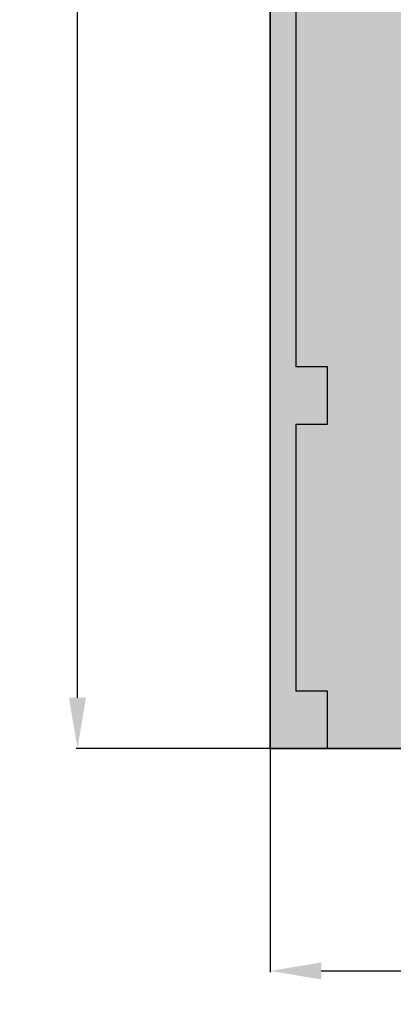
# Model space of a CAD drawing. Units: inches. Extents: x 389 to 971, y 148 to 870.
# Tile 1 of 14: x 389 to 448, y 194 to 349. Entities that reach past the tile are written whole.
import ezdxf

# ---------------------------------------------------------------- set-up
doc = ezdxf.new("R2010")
doc.units = ezdxf.units.IN
doc.header["$MEASUREMENT"] = 0
for name, color, linetype, lineweight in [('A-ANNO-DIMS', 2, 'Continuous', 18), ('C-PROP', 7, 'Continuous', 35), ('L-GATE', 4, 'Continuous', 25), ('L-GRND-BASE-PATT', 8, 'Continuous', 13), ('L-WALL', 7, 'Continuous', 30)]:
    doc.layers.add(name, color=color, linetype=linetype, lineweight=lineweight)
for name, color, linetype, lineweight, true_color in [('A-WALL-PATT', 18, 'Continuous', 13, 0x000000), ('L-GRND-PATT', 39, 'Continuous', 13, 0x603913), ('L-WALL-PATT', 18, 'Continuous', 13, 0x000000)]:
    doc.layers.add(name, color=color, linetype=linetype, lineweight=lineweight, true_color=true_color)
doc.styles.get("Standard").update_dxf_attribs({"font": 'arial.ttf'})
doc.dimstyles.get("Standard").update_dxf_attribs({"dimtxt": 8, "dimasz": 8, "dimexe": 0.18, "dimexo": 0.0625, "dimgap": 0.09, "dimtad": 0, "dimtih": 1, "dimtoh": 1, "dimdec": 0, "dimzin": 0, "dimdsep": 46, "dimlunit": 3, "dimtxsty": 'Standard', "dimcen": 0.09, "dimadec": 0, "dimazin": 0, "dimtfac": 1, "dimtdec": 0, "dimtofl": 0, "dimtmove": 0, "dimatfit": 3, "dimfxl": 1, "dimtolj": 1, "dimtzin": 0, "dimarcsym": 0})

# ---------------------------------------------------------------- blocks, each defined once
blk = doc.blocks.new('*D44')
at = {"layer": 'A-ANNO-DIMS', "color": 0, "lineweight": -2, "transparency": 16777216}
for p, q in [((428.216024, 234.582013), (428.216024, 199.495293)), ((848.2160239999998, 234.582013), (848.2160239999998, 199.495293)), ((436.216024, 199.675293), (629.1410308212824, 199.675293)), ((840.2160239999998, 199.675293), (647.2910171787175, 199.675293))]:
    blk.add_line(p, q, dxfattribs=at)
at = {"layer": 'A-ANNO-DIMS', "color": 0, "transparency": 16777216}
for points in [[(436.216024, 201.0086263333334), (436.216024, 198.3419596666666), (428.216024, 199.675293)], [(840.2160239999998, 201.0086263333334), (840.2160239999998, 198.3419596666666), (848.2160239999998, 199.675293)]]:
    blk.add_solid(points, dxfattribs=at)
at = {"layer": 'Defpoints', "color": 0, "transparency": 16777216}
for p in [(428.216024, 234.644513), (848.2160239999998, 234.644513), (848.2160239999998, 199.675293)]:
    blk.add_point(p, dxfattribs=at)
at = {"layer": 'A-ANNO-DIMS', "color": 0, "transparency": 16777216, "insert": (638.216024, 199.675293), "char_height": 8, "attachment_point": 5}
blk.add_mtext('\\A1;420', dxfattribs=at)
blk = doc.blocks.new('*D45')
at = {"layer": 'A-ANNO-DIMS', "color": 0, "lineweight": -2, "transparency": 16777216}
for p, q in [((428.1535240000002, 834.6445130000004), (397.7110240000004, 834.6445130000004)), ((397.8910240000004, 826.6445130000004), (397.8910240000005, 538.8190969017736)), ((397.8910240000005, 242.6445130000001), (397.8910240000005, 530.4699290982267)), ((428.1535240000002, 234.6445130000001), (397.7110240000005, 234.6445130000001))]:
    blk.add_line(p, q, dxfattribs=at)
at = {"layer": 'A-ANNO-DIMS', "color": 0, "transparency": 16777216}
for points in [[(396.5576906666671, 826.6445130000004), (399.2243573333337, 826.6445130000004), (397.8910240000004, 834.6445130000004)], [(396.5576906666672, 242.6445130000001), (399.2243573333338, 242.6445130000001), (397.8910240000005, 234.6445130000001)]]:
    blk.add_solid(points, dxfattribs=at)
at = {"layer": 'Defpoints', "color": 0, "transparency": 16777216}
for p in [(397.8910240000004, 834.6445130000004), (428.2160240000002, 834.6445130000004), (428.2160240000002, 234.6445130000001)]:
    blk.add_point(p, dxfattribs=at)
at = {"layer": 'A-ANNO-DIMS', "color": 0, "transparency": 16777216, "insert": (397.8910240000005, 534.6445129999998), "char_height": 8, "attachment_point": 5}
blk.add_mtext('\\A1;600', dxfattribs=at)

msp = doc.modelspace()

# ---------------------------------------------------------------- hatches: boundary and pattern name
at = {"layer": 'A-WALL-PATT'}
h = msp.add_hatch(color=256, dxfattribs=at)
h.dxf.hatch_style = 1
h.paths.add_polyline_path([(432.2160244416713, 434.6445131961097), (436.3672936601142, 434.6445131961097), (436.3672936601142, 443.6445131961098), (432.2160244416713, 443.6445131961098), (432.2160244416714, 830.6445131961094), (746.2160244416714, 830.6445131961098), (746.2160244416714, 823.8175070811654), (755.2160244416712, 823.8175070811657), (755.2160244416712, 825.6445131961098), (839.2160244416713, 825.6445131961098), (839.2160244416713, 803.5176064986067), (839.2160244416712, 741.6445131961098), (755.2160244416712, 741.6445131961098), (755.2160244416712, 748.4596256139029), (755.1858732057922, 748.4596256139029), (750.7160244416712, 748.4596256139029), (746.2160244416714, 748.4596256139029), (746.2160244416714, 732.6445131961098), (839.2160244416712, 732.6445131961098), (839.2160244416712, 600.6445131961098), (708.5170970640701, 600.6445131961098), (708.5170970640701, 596.1445131961098), (708.5170970640701, 591.6445131961098), (794.2160244416712, 591.6445131961098), (794.2160244416712, 587.4291281246713), (803.2160244416712, 587.4291281246713), (803.2160244416712, 591.6445131961098), (839.2160244416712, 591.6445131961098), (839.2160244416712, 466.6011988194286), (803.2160244416712, 466.6011988194285), (803.2160244416712, 471.0308934694551), (794.2160244416712, 471.0308934694551), (794.2160244416712, 466.6011988194285), (784.6144969105871, 466.6011988194285), (784.6144969105871, 457.6011988194286), (839.2160244416712, 457.6011988194286), (839.2160244416712, 447.6445131961096), (839.2160244416713, 294.6445131961098), (810.0513609197294, 294.6445131961098), (810.0513609197296, 285.6445131961097), (839.2160244416713, 285.6445131961097), (839.2160244416713, 238.6445131961098), (590.2160244416713, 238.6445131961097), (590.2160244416713, 234.6445131961098), (848.2160244416714, 234.6445131961098), (848.2160244416714, 834.6445131961098), (428.2160244416714, 834.6445131961098), (428.2160244416714, 234.6445131961098), (437.2160244416714, 234.6445131961098), (437.2160244416714, 243.6445131961098), (432.2160244416713, 243.6445131961098)])
at = {"layer": 'L-GRND-BASE-PATT'}
h = msp.add_hatch(color=256, dxfattribs=at)
h.dxf.hatch_style = 1
edge = h.paths.add_edge_path(flags=16)
edge.add_ellipse((8782.002602781105, 354.2472542798386), major_axis=(-8296.949265805946, 5.39345e-11), ratio=0.8423038695428886, start_angle=-0.0902290885933894, end_angle=0.3838667787920258, ccw=False)
edge.add_ellipse((485.0533369751568, 368.2895347624687), major_axis=(-1.159084047334488, 1.838e-13), ratio=0.8423038695439892, start_angle=9.094947017729282e-12, end_angle=90.00000000000898, ccw=False)
edge.add_line((483.8942529278224, 368.2895347624687), (483.8942529278225, 387.6039063360424))
edge.add_ellipse((485.0533369751571, 387.2465553762829), major_axis=(1.159084047334488, 1.838e-13), ratio=0.8423038695439892, start_angle=89.99999999999102, end_angle=179.9999999999909, ccw=False)
edge.add_line((485.0533369751572, 388.2228563544795), (485.5047440247956, 388.2228563544795))
edge.add_ellipse((898.8202485054873, 372.489720535918), major_axis=(413.7373561031672, 1.26113e-11), ratio=0.8423038695441164, start_angle=176.3495724142986, end_angle=177.8200496863524, ccw=False)
edge.add_ellipse((535.9119176052733, 196.3854951855018), major_axis=(-245.3971626940985, 1.013648e-10), ratio=0.8423038695442548, start_angle=-77.87403444769302, end_angle=-76.2194710104792, ccw=False)
edge.add_ellipse((535.9119176052684, 201.7546502845751), major_axis=(239.1273775699096, 1.008988e-10), ratio=0.842303869543627, start_angle=100.20953899711827, end_angle=102.44462729341922, ccw=False)
edge.add_ellipse((473.3138688667988, 564.9222417143382), major_axis=(196.5636751472093, 8.4793e-12), ratio=0.8423038695439335, start_angle=-80.74343399280163, end_angle=-77.44506735586587)
edge.add_line((509.5535496243029, 402.1940957519602), (514.3535105156315, 404.8483349684994))
edge.add_line((514.3535105156315, 404.8483349684994), (514.3535105156315, 404.7971763262221))
edge.add_ellipse((514.3535105156316, 404.2643898676136), major_axis=(0.5795420236673633, 2e-16), ratio=0.8423038695437671, start_angle=52.06686954015339, end_angle=90.00000000001342, ccw=False)
edge.add_line((514.671564037824, 404.672460591463), (519.1534714069603, 402.19409575196))
edge.add_ellipse((555.3931521644682, 564.9222417143374), major_axis=(-196.5636751472384, 3.62381e-11), ratio=0.8423038695438114, start_angle=77.44506735587258, end_angle=80.74343399280833)
edge.add_ellipse((492.795103425985, 201.7546502845724), major_axis=(239.12737756976, 4.82267e-11), ratio=0.8423038695441539, start_angle=77.55537270654253, end_angle=79.7904610028433, ccw=False)
edge.add_ellipse((492.7951034259847, 196.3854951855023), major_axis=(245.3971626940514, 1.422861e-10), ratio=0.8423038695444116, start_angle=76.21947101046823, end_angle=77.87403444768199, ccw=False)
edge.add_ellipse((129.8867725257751, 372.4897205359271), major_axis=(-413.7373561031673, 2.44623e-11), ratio=0.8423038695441432, start_angle=182.179950313648, end_angle=183.6504275857018, ccw=False)
edge.add_line((543.2022770064673, 388.2228563544788), (544.0779382625514, 388.2228563544787))
edge.add_ellipse((543.6536840561057, 387.2465553762822), major_axis=(-1.159084047334545, 1.527e-13), ratio=0.8423038695438989, start_angle=180.0000000000075, end_angle=270.00000000000756, ccw=False)
edge.add_line((544.8127681034401, 387.2465553762826), (544.8127681034399, 367.9321838027083))
edge.add_ellipse((543.6536840561054, 368.2895347624679), major_axis=(1.159084047334544, 7.24e-14), ratio=0.8423038695439478, start_angle=269.9999999999964, end_angle=359.9999999999964, ccw=False)
edge.add_ellipse((-7753.295581726658, 354.2472542799028), major_axis=(-8296.949265782761, 2.068448e-10), ratio=0.8423038695442414, start_angle=179.6161332212083, end_angle=180.0902290885951, ccw=False)
edge.add_line((543.3912265319653, 298.6607849184036), (544.0779382625504, 298.6607849184036))
edge.add_ellipse((543.6536840561046, 297.6844839402071), major_axis=(1.159084047334431, 1.769e-13), ratio=0.8423038695439814, start_angle=-1.1482370609883219e-11, end_angle=89.99999999999119, ccw=False)
edge.add_line((544.8127681034391, 297.684483940207), (544.8127681034387, 278.3701123666333))
edge.add_ellipse((543.6536840561043, 278.727463326393), major_axis=(-1.159084047334431, 2.574e-13), ratio=0.8423038695440306, start_angle=90.00000000001268, end_angle=180.0000000000099, ccw=False)
edge.add_line((543.6536840561045, 277.7511623481965), (543.1566278692261, 277.7511623481965))
edge.add_ellipse((-7753.295581726658, 354.2472542799028), major_axis=(-8296.949265782761, 2.068448e-10), ratio=0.8423038695442414, start_angle=179.3813568036816, end_angle=179.4717285281829, ccw=False)
edge.add_ellipse((542.4236240941387, 263.2762864208561), major_axis=(-1.738626071001761, 2.132e-13), ratio=0.8423038695439151, start_angle=179.3717627838137, end_angle=248.464756601011, ccw=False)
edge.add_ellipse((-7753.875123750511, 354.2472542780016), major_axis=(-8298.740341433751, 2.4782644722e-06), ratio=0.8423038662721074, start_angle=179.3534459200609, end_angle=179.3717628008941, ccw=False)
edge.add_ellipse((540.0116322079951, 260.6509346628677), major_axis=(-4.109243751168186, 2.384e-13), ratio=0.842303869543976, start_angle=90.0000000000635, end_angle=179.3534459029233, ccw=False)
edge.add_line((540.0116322079991, 257.1897027503593), (488.6953888232593, 257.1897027503609))
edge.add_ellipse((488.6953888232669, 260.6509346628715), major_axis=(4.10924375117072, 1.262e-13), ratio=0.8423038695439824, start_angle=180.6465540970565, end_angle=269.9999999998589, ccw=False)
edge.add_ellipse((8782.582144816053, 354.2472542821698), major_axis=(-8298.740341477976, 1.8591886369e-06), ratio=0.8423038720186145, start_angle=0.6282372290784792, end_angle=0.6465541099116194, ccw=False)
edge.add_ellipse((486.2833969371199, 263.2762864208594), major_axis=(-1.738626071002378, 2.7e-13), ratio=0.8423038695439394, start_angle=-68.46475649596817, end_angle=0.6282372161796275, ccw=False)
edge.add_ellipse((8782.002602781105, 354.2472542798386), major_axis=(-8296.949265805946, 5.39345e-11), ratio=0.8423038695428886, start_angle=0.5282714718171064, end_angle=0.6465540970606867, ccw=False)
edge.add_line((485.5503931620382, 277.7511623481972), (484.6290827687102, 277.7511623481972))
edge.add_ellipse((485.0533369751559, 278.7274633263938), major_axis=(-1.159084047334545, 3.11e-13), ratio=0.8423038695439968, start_angle=1.5404566511278972e-11, end_angle=90.000000000012, ccw=False)
edge.add_line((483.8942529278214, 278.7274633263938), (483.8942529278216, 298.0418348999672))
edge.add_ellipse((485.053336975156, 297.6844839402078), major_axis=(1.159084047334488, 1.025e-13), ratio=0.8423038695440382, start_angle=89.99999999999488, end_angle=179.9999999999949, ccw=False)
edge = h.paths.add_edge_path(flags=0)
edge.add_ellipse((8782.002602781096, 354.247254279773), major_axis=(-8295.790181758603, 9.87839e-10), ratio=0.8423038695486498, start_angle=0.05559431350519617, end_angle=0.37776419391582294, ccw=False)
edge.add_line((486.2179253655185, 346.1978202249628), (489.3905023836935, 335.8383575186984))
edge.add_ellipse((3386.011413077446, 329.726312794031), major_axis=(-2896.629999631248, 1.069454e-10), ratio=0.8423038695494893, start_angle=-0.1208973690315206, end_angle=0.3640763488915184)
edge.add_line((489.4638383140943, 311.3204429697198), (486.4665645878948, 299.5520931219791))
edge = h.paths.add_edge_path(flags=0)
edge.add_ellipse((514.3535105156315, 391.3730654902235), major_axis=(-115.1512533244504, 1.8736e-12), ratio=0.8423038695439684, start_angle=76.4018653097696, end_angle=103.5981346902308)
edge.add_line((537.3427693057832, 296.3333211885938), (537.342769305783, 281.5897392316151))
edge.add_ellipse((514.3535105156313, 376.6294835332447), major_axis=(-115.1512533244486, 9.02e-13), ratio=0.8423038695439828, start_angle=76.40186530976922, end_angle=103.59813469023032, ccw=False)
edge.add_line((491.3642517254773, 281.5897392316156), (491.3642517254774, 296.3333211885945))
edge = h.paths.add_edge_path(flags=0)
edge.add_line((491.3642517254777, 337.0752369161334), (489.6529508739416, 349.9015767089268))
edge.add_ellipse((510.1338164488795, 298.7862183048575), major_axis=(64.04807894948699, 3.9006e-12), ratio=0.8423038695439252, start_angle=94.27742096304979, end_angle=111.83495379670401, ccw=False)
edge.add_line((506.106812905481, 352.6274231954524), (522.600208125781, 352.6274231954521))
edge.add_ellipse((518.5732045823798, 298.7862183048586), major_axis=(64.04807894948067, 3.24e-14), ratio=0.8423038695439885, start_angle=68.16504620328948, end_angle=85.72257903694378, ccw=False)
edge.add_line((539.05407015732, 349.9015767089259), (537.3427693057835, 337.0752369161327))
edge.add_ellipse((516.5461636849332, 287.5825181681899), major_axis=(62.33048198262021, 1.5954e-12), ratio=0.8423038695439995, start_angle=67.20808512240782, end_angle=85.12993040286212)
edge.add_line((521.0080028322477, 339.9490379899644), (507.6990181990146, 339.9490379899646))
edge.add_ellipse((512.1608573463288, 287.5825181681774), major_axis=(62.33048198263887, 2.0798e-12), ratio=0.8423038695439498, start_angle=94.8700695971331, end_angle=112.791914877584)
edge = h.paths.add_edge_path(flags=0)
edge.add_ellipse((493.6824198201462, 273.9438556676354), major_axis=(-2.318168094668919, 1.896e-13), ratio=0.8423038695439611, start_angle=-89.99999999999523, end_angle=4.718003765447065e-12, ccw=False)
edge.add_line((493.6824198201462, 275.8964576240284), (535.3743409680425, 275.8964576240277))
edge.add_ellipse((535.024601211114, 273.9438556676347), major_axis=(2.318168094668976, 2.946e-13), ratio=0.8423038695439647, start_angle=-7.275957614183426e-12, end_angle=89.99999999998943, ccw=False)
edge.add_line((537.342769305783, 273.9438556676347), (537.3427693057827, 258.698332706474))
edge.add_line((537.3427693057827, 258.698332706474), (540.5911742316662, 258.6983327064739))
edge.add_ellipse((540.5911742316634, 260.6509346628669), major_axis=(-2.318168094668839, 2.143e-13), ratio=0.8423038695440144, start_angle=90.00000000008203, end_angle=179.3534459029346)
edge.add_line((540.5911742316662, 258.6983327064739), (487.7691399811528, 258.6983327064755))
edge.add_ellipse((488.1158467995968, 260.6509346628684), major_axis=(2.318168094668909, 7.48e-14), ratio=0.8423038695439647, start_angle=180.6465540970884, end_angle=269.9999999999081)
edge.add_line((488.1158467995931, 258.6983327064755), (491.3642517254771, 258.6983327064754))
edge.add_line((491.3642517254771, 258.6983327064754), (491.3642517254771, 274.2384428182294))
h.paths.add_polyline_path([(746.1375687288224, 327.3223047166553), (750.1400147212453, 327.3223047166553), (750.1400147212453, 326.2830696147227), (798.1693712998389, 326.2830696147227), (798.1693712998389, 327.3223047166553), (802.1718172922616, 327.3223047166553), (802.1718172922616, 309.9783792024682, -0.1904762075443491), (746.1375687288224, 309.9783668090107)], flags=16)
h.paths.add_polyline_path([(782.1595875801748, 313.5684994305933), (782.1595893317732, 309.0414930416419, -0.0496282101666581), (766.1497986905329, 309.0414910503953), (766.1498004421323, 313.5684994305933)], flags=0)
h.paths.add_polyline_path([(755.1858908233534, 344.9352232902417), (755.1858908233534, 373.916311072083), (788.1243995226009, 373.916311072083), (788.1243995226009, 344.9352232902417)], flags=16)
h.paths.add_polyline_path([(757.1858908233535, 346.9352232902417), (757.1858908233535, 371.916311072083), (786.1243995226009, 371.916311072083), (786.1243995226009, 346.9352232902417)], flags=0)
h.paths.add_polyline_path([(803.6445810111745, 338.4878931208803), (803.6445810111745, 342.4903391133031), (804.6838161131072, 342.4903391133031), (804.6838161131072, 390.5196956918968), (803.6445810111748, 390.5196956918968), (803.6445810111748, 394.5221416843196), (820.9885065253617, 394.5221416843196, -0.1904762075443491), (820.9885189188192, 338.4878931208803)], flags=16)
h.paths.add_polyline_path([(806.8706930931005, 326.6963103558256), (806.4254411777042, 327.1415622712219), (806.4723791864895, 326.6297175483474)], flags=16)
h.paths.add_polyline_path([(822.0328146004263, 317.4007976138144), (822.1941503181826, 317.8932883068639), (821.562628166435, 317.9885306563034)], flags=16)
h.paths.add_polyline_path([(817.3983862972365, 358.5001248341902), (817.3983862972365, 374.5099119722327), (821.9253926861879, 374.5099137238312, -0.049628210166658), (821.9253946774346, 358.5001230825909)], flags=0)
h.paths.add_polyline_path([(808.1446344648577, 418.9736619306146), (808.2246858861593, 418.5632188717996), (808.5395491501399, 418.5787472453325)], flags=16)
h.paths.add_polyline_path([(820.3158762739024, 412.6690288868844), (820.4772119916585, 413.161519579934), (819.8456898399113, 413.2567619293735)], flags=16)
h.paths.add_polyline_path([(466.3155093563569, 235.5246322146605), (517.3806533266912, 235.5246322146605), (517.3806533266912, 244.4269231682286), (466.3155093563569, 244.4269231682286)], flags=24)
h.paths.add_polyline_path([(739.8737195480014, 256.2000079819968), (815.4040239338423, 256.2000079819968), (815.4040239338423, 265.3453807094367), (739.8737195480014, 265.3453807094367)], flags=24)
h.paths.add_polyline_path([(750.6081538187397, 393.6666679930368), (791.5680640722773, 393.6666679930368), (791.5680640722773, 412.3933175868746), (750.6081538187397, 412.3933175868746)], flags=24)
h.paths.add_polyline_path([(438.9630812812552, 410.0618566955462), (484.6203810968238, 410.0618566955462), (484.6203810968238, 429.1217352891893), (438.9630812812552, 429.1217352891893)], flags=24)
edge = h.paths.add_edge_path()
edge.add_line((839.2160244416713, 285.6445131961097), (611.8786784019748, 285.6445131961099))
edge.add_line((611.8786784019748, 285.6445131961099), (604.3870116090119, 285.6445131961097))
edge.add_line((604.3870116090119, 285.6445131961097), (595.3870116090119, 285.6445131961097))
edge.add_line((595.3870116090119, 285.6445131961097), (595.3870116090118, 370.1553848722774))
edge.add_line((595.3870116090118, 370.1553848722774), (604.0816928471932, 370.1553848722774))
edge.add_line((604.0816928471932, 370.1553848722774), (604.0816928471932, 371.3788335667469))
edge.add_line((604.0816928471932, 371.3788335667469), (632.0194586761203, 371.3788335667469))
edge.add_arc((604.0816928471932, 370.1553848722773), 27.96454158787471, 2.507490703587644, 90.00000000000003)
edge.add_line((604.0816928471932, 398.1199264601519), (599.8870116090108, 398.1652144688576))
edge.add_line((599.8870116090108, 398.1652144688576), (604.4225424425357, 398.1652144688576))
edge.add_arc((604.4225424425357, 428.4020866923496), 30.23687222349201, 270.0000000000002, 357.492509296413)
edge.add_line((634.6304631740308, 427.0792235325719), (604.4225424425357, 427.0792235325719))
edge.add_line((604.4225424425357, 427.0792235325719), (604.4225424425357, 428.4020866923497))
edge.add_line((604.4225424425357, 428.4020866923497), (599.8870116090119, 428.4020866923497))
edge.add_line((599.8870116090119, 428.4020866923497), (595.3870116090116, 428.4020866923497))
edge.add_line((595.3870116090116, 428.4020866923497), (595.3870116090118, 434.6445131961097))
edge.add_line((595.3870116090118, 434.6445131961097), (585.0790669792458, 434.6445131961097))
edge.add_line((585.0790669792458, 434.6445131961097), (540.3921730610418, 434.6445131961097))
edge.add_line((540.3921730610418, 434.6445131961097), (526.712508448134, 434.6445131961097))
edge.add_line((526.712508448134, 434.6445131961097), (488.4094553949635, 434.6445131961097))
edge.add_line((488.4094553949635, 434.6445131961097), (432.2160244416713, 434.6445131961097))
edge.add_line((432.2160244416713, 434.6445131961097), (432.2160244416713, 243.6445131961098))
edge.add_line((432.2160244416713, 243.6445131961098), (437.2160244416714, 243.6445131961098))
edge.add_line((437.2160244416714, 243.6445131961098), (437.2160244416714, 234.6445131961098))
edge.add_line((437.2160244416714, 234.6445131961098), (581.2160244416713, 234.6445131961098))
edge.add_line((581.2160244416713, 234.6445131961098), (581.2160244416713, 238.6445131961097))
edge.add_line((581.2160244416713, 238.6445131961097), (581.2160244416713, 243.6445131961098))
edge.add_line((581.2160244416713, 243.6445131961098), (590.2160244416713, 243.6445131961098))
edge.add_line((590.2160244416713, 243.6445131961098), (590.2160244416713, 238.6445131961097))
edge.add_line((590.2160244416713, 238.6445131961097), (839.2160244416713, 238.6445131961098))
edge.add_line((839.2160244416713, 238.6445131961098), (839.2160244416713, 285.6445131961097))
at = {"layer": 'L-GRND-PATT'}
h = msp.add_hatch(dxfattribs=at)
h.set_pattern_fill('EARTH', color=256, angle=45)
h.set_pattern_definition([(45, (0, 0), (0, 8.980256121069154), [6.349999999999999, -6.349999999999999]), (45, (-1.683798022700466, 1.683798022700466), (0, 8.980256121069154), [6.349999999999999, -6.349999999999999]), (45, (-3.367596045400933, 3.367596045400933), (0, 8.980256121069154), [6.349999999999999, -6.349999999999999]), (135, (-3.367596045400933, 4.490128060534576), (-8.980256121069154, 0), [6.349999999999999, -6.349999999999999]), (135, (-1.683798022700466, 6.173926083235043), (-8.980256121069154, 0), [6.349999999999999, -6.349999999999999]), (135, (0, 7.85772410593551), (-8.980256121069154, 0), [6.349999999999999, -6.349999999999999])])
h.paths.add_polyline_path([(432.2160244416713, 243.6445131961098), (437.2160244416714, 243.6445131961098), (437.2160244416714, 234.6445131961098), (581.2160244416713, 234.6445131961098), (581.2160244416713, 238.6445131961097), (581.2160244416713, 243.6445131961098), (590.2160244416713, 243.6445131961098), (590.2160244416713, 238.6445131961097), (839.2160244416713, 238.6445131961098), (839.2160244416712, 285.6445131961097), (810.0513609197296, 285.6445131961097), (733.8056934525983, 285.6445131961099), (684.2433676403508, 285.6445131961098), (611.8786784019748, 285.6445131961099), (604.3870116090119, 285.6445131961097), (595.3870116090119, 285.6445131961097), (595.3870116090118, 370.1553848722774), (604.0816928471932, 370.1553848722774), (604.0816928471932, 371.3788335667469), (632.0194586761203, 371.3788335667469, 0.4014527144963568), (604.0816928471932, 398.119926460152), (599.8870116090127, 398.1652144688576), (604.4225424425357, 398.1652144688576, 0.4014527144963579), (634.6304631740308, 427.0792235325719), (604.4225424425357, 427.0792235325719), (604.4225424425357, 428.4020866923497), (599.8870116090119, 428.4020866923497), (595.3870116090116, 428.4020866923497), (595.3870116090118, 434.6445131961097), (585.0790669792458, 434.6445131961097), (540.3921730610418, 434.6445131961097), (526.712508448134, 434.6445131961097), (488.4094553949635, 434.6445131961097), (432.2160244416713, 434.6445131961097)])
edge = h.paths.add_edge_path(flags=16)
edge.add_line((483.8942529278214, 278.7274633263938), (483.8942529278216, 298.2563878122772))
edge.add_ellipse((485.053336975156, 297.6844839402078), major_axis=(1.159084047334488, 1.025e-13), ratio=0.8423038695440382, start_angle=89.99999999999488, end_angle=179.9999999999949, ccw=False)
edge.add_ellipse((8782.002602781105, 354.2472542798386), major_axis=(-8296.949265805946, 5.39345e-11), ratio=0.8423038695428886, start_angle=-0.0902290885933894, end_angle=0.3838667787920258, ccw=False)
edge.add_ellipse((485.0533369751568, 368.2895347624687), major_axis=(-1.159084047334488, 1.838e-13), ratio=0.8423038695439892, start_angle=9.094947017729282e-12, end_angle=90.00000000000898, ccw=False)
edge.add_line((483.8942529278224, 368.2895347624687), (483.8942529278225, 387.8184592483523))
edge.add_ellipse((485.0533369751571, 387.2465553762829), major_axis=(1.159084047334488, 1.838e-13), ratio=0.8423038695439892, start_angle=89.99999999999102, end_angle=179.9999999999909, ccw=False)
edge.add_ellipse((898.8202485054873, 372.489720535918), major_axis=(413.7373561031672, 1.26113e-11), ratio=0.8423038695441164, start_angle=176.3495724142986, end_angle=177.8200496863524, ccw=False)
edge.add_ellipse((535.9119176052733, 196.3854951855018), major_axis=(-245.3971626940985, 1.013648e-10), ratio=0.8423038695442548, start_angle=-77.87403444769302, end_angle=-76.2194710104792, ccw=False)
edge.add_ellipse((535.9119176052684, 201.7546502845751), major_axis=(239.1273775699096, 1.008988e-10), ratio=0.842303869543627, start_angle=100.20953899711827, end_angle=102.44462729341922, ccw=False)
edge.add_ellipse((473.3138688667988, 564.9222417143382), major_axis=(196.5636751472093, 8.4793e-12), ratio=0.8423038695439335, start_angle=-80.74343399280163, end_angle=-77.44506735586587)
edge.add_line((509.5535496243029, 402.1940957519602), (514.3535105156316, 404.8483349684994))
edge.add_line((514.3535105156316, 404.8483349684994), (519.1534714069603, 402.19409575196))
edge.add_ellipse((555.3931521644682, 564.9222417143374), major_axis=(-196.5636751472384, 3.62381e-11), ratio=0.8423038695438114, start_angle=77.44506735587258, end_angle=80.74343399280833)
edge.add_ellipse((492.795103425985, 201.7546502845724), major_axis=(239.12737756976, 4.82267e-11), ratio=0.8423038695441539, start_angle=77.55537270654253, end_angle=79.7904610028433, ccw=False)
edge.add_ellipse((492.7951034259847, 196.3854951855023), major_axis=(245.3971626940514, 1.422861e-10), ratio=0.8423038695444116, start_angle=76.21947101046823, end_angle=77.87403444768199, ccw=False)
edge.add_ellipse((129.8867725257751, 372.4897205359271), major_axis=(-413.7373561031673, 2.44623e-11), ratio=0.8423038695441432, start_angle=182.179950313648, end_angle=183.6504275857018, ccw=False)
edge.add_line((543.2022770064673, 388.2228563544789), (544.3326597711041, 388.2228563544786))
edge.add_ellipse((543.6536840561057, 387.2465553762822), major_axis=(-1.159084047334545, 1.527e-13), ratio=0.8423038695438989, start_angle=180.0000000000075, end_angle=270.00000000000756, ccw=False)
edge.add_line((544.8127681034401, 387.2465553762825), (544.8127681034399, 367.7176308903986))
edge.add_ellipse((543.6536840561054, 368.2895347624679), major_axis=(1.159084047334544, 7.24e-14), ratio=0.8423038695439478, start_angle=269.9999999999964, end_angle=359.9999999999964, ccw=False)
edge.add_ellipse((-7753.295581726658, 354.2472542799028), major_axis=(-8296.949265782761, 2.068448e-10), ratio=0.8423038695442414, start_angle=179.6161332212083, end_angle=180.0902290885951, ccw=False)
edge.add_ellipse((543.6536840561046, 297.6844839402071), major_axis=(1.159084047334431, 1.769e-13), ratio=0.8423038695439814, start_angle=-1.1482370609883219e-11, end_angle=89.99999999999119, ccw=False)
edge.add_line((544.8127681034391, 297.6844839402071), (544.8127681034387, 278.1555594543235))
edge.add_ellipse((543.6536840561043, 278.727463326393), major_axis=(-1.159084047334431, 2.574e-13), ratio=0.8423038695440306, start_angle=90.00000000001268, end_angle=180.0000000000099, ccw=False)
edge.add_ellipse((-7753.295581726658, 354.2472542799028), major_axis=(-8296.949265782761, 2.068448e-10), ratio=0.8423038695442414, start_angle=179.3813568036816, end_angle=179.4717285281829, ccw=False)
edge.add_ellipse((542.4236240941387, 263.2762864208561), major_axis=(-1.738626071001761, 2.132e-13), ratio=0.8423038695439151, start_angle=179.3717627838137, end_angle=248.464756601011, ccw=False)
edge.add_ellipse((-7753.875123750511, 354.2472542780016), major_axis=(-8298.740341433751, 2.4782644722e-06), ratio=0.8423038662721074, start_angle=179.3534459200609, end_angle=179.3717628008941, ccw=False)
edge.add_ellipse((540.0116322079951, 260.6509346628677), major_axis=(-4.109243751168186, 2.384e-13), ratio=0.842303869543976, start_angle=90.0000000000635, end_angle=179.3534459029233, ccw=False)
edge.add_line((540.0116322079989, 257.1897027503593), (488.0808074948215, 257.1897027503609))
edge.add_ellipse((488.6953888232669, 260.6509346628715), major_axis=(4.10924375117072, 1.262e-13), ratio=0.8423038695439824, start_angle=180.6465540970565, end_angle=269.9999999998589, ccw=False)
edge.add_ellipse((8782.582144816053, 354.2472542821698), major_axis=(-8298.740341477976, 1.8591886369e-06), ratio=0.8423038720186145, start_angle=0.6282372290784792, end_angle=0.6465541099116194, ccw=False)
edge.add_ellipse((486.2833969371199, 263.2762864208594), major_axis=(-1.738626071002378, 2.7e-13), ratio=0.8423038695439394, start_angle=-68.46475649596817, end_angle=0.6282372161796275, ccw=False)
edge.add_ellipse((8782.002602781105, 354.2472542798386), major_axis=(-8296.949265805946, 5.39345e-11), ratio=0.8423038695428886, start_angle=0.5282714718171064, end_angle=0.6465540970606867, ccw=False)
edge.add_line((485.5503931620382, 277.7511623481972), (484.3743612601578, 277.7511623481972))
edge.add_ellipse((485.0533369751559, 278.7274633263938), major_axis=(-1.159084047334545, 3.11e-13), ratio=0.8423038695439968, start_angle=1.5404566511278972e-11, end_angle=90.000000000012, ccw=False)
edge = h.paths.add_edge_path(flags=0)
edge.add_ellipse((488.1158467995968, 260.6509346628684), major_axis=(2.318168094668909, 7.48e-14), ratio=0.8423038695439647, start_angle=180.6465540970884, end_angle=269.9999999999081)
edge.add_line((488.1158467995933, 258.6983327064755), (491.3642517254771, 258.6983327064753))
edge.add_line((491.3642517254771, 258.6983327064753), (491.3642517254771, 274.4686391213292))
edge.add_ellipse((493.6824198201462, 273.9438556676354), major_axis=(-2.318168094668919, 1.896e-13), ratio=0.8423038695439611, start_angle=-89.99999999999523, end_angle=4.718003765447065e-12, ccw=False)
edge.add_line((493.6824198201462, 275.8964576240284), (535.6476346230087, 275.8964576240277))
edge.add_ellipse((535.024601211114, 273.9438556676347), major_axis=(2.318168094668976, 2.946e-13), ratio=0.8423038695439647, start_angle=-7.275957614183426e-12, end_angle=89.99999999998943, ccw=False)
edge.add_line((537.342769305783, 273.9438556676347), (537.3427693057827, 258.698332706474))
edge.add_line((537.3427693057827, 258.698332706474), (541.2086129152347, 258.6983327064739))
edge.add_ellipse((540.5911742316634, 260.6509346628669), major_axis=(-2.318168094668839, 2.143e-13), ratio=0.8423038695440144, start_angle=90.00000000008203, end_angle=179.3534459029347, ccw=False)
edge.add_line((540.5911742316662, 258.6983327064739), (487.4984081160257, 258.6983327064755))
edge = h.paths.add_edge_path(flags=0)
edge.add_line((491.3642517254773, 281.5897392316156), (491.3642517254774, 296.3333211885945))
edge.add_ellipse((514.3535105156315, 391.3730654902235), major_axis=(-115.1512533244504, 1.8736e-12), ratio=0.8423038695439684, start_angle=76.4018653097696, end_angle=103.5981346902308)
edge.add_line((537.3427693057832, 296.3333211885938), (537.342769305783, 281.5897392316151))
edge.add_ellipse((514.3535105156313, 376.6294835332447), major_axis=(-115.1512533244486, 9.02e-13), ratio=0.8423038695439828, start_angle=76.40186530976922, end_angle=103.59813469023032, ccw=False)
edge = h.paths.add_edge_path(flags=0)
edge.add_ellipse((8782.002602781096, 354.247254279773), major_axis=(-8295.790181758603, 9.87839e-10), ratio=0.8423038695486498, start_angle=0.05559431350519617, end_angle=0.37776419391582294, ccw=False)
edge.add_line((486.2179253655185, 346.1978202249628), (489.3905023836935, 335.8383575186985))
edge.add_ellipse((3386.011413077446, 329.726312794031), major_axis=(-2896.629999631248, 1.069454e-10), ratio=0.8423038695494893, start_angle=-0.1208973690315206, end_angle=0.3640763488915184)
edge.add_line((489.4638383140943, 311.3204429697198), (486.4665645878948, 299.5520931219782))
edge = h.paths.add_edge_path(flags=0)
edge.add_line((491.3642517254777, 337.0752369161334), (489.6529508739416, 349.9015767089268))
edge.add_ellipse((510.1338164488795, 298.7862183048575), major_axis=(64.04807894948699, 3.9006e-12), ratio=0.8423038695439252, start_angle=94.27742096304979, end_angle=111.83495379670401, ccw=False)
edge.add_line((506.106812905481, 352.6274231954524), (522.600208125781, 352.6274231954521))
edge.add_ellipse((518.5732045823798, 298.7862183048586), major_axis=(64.04807894948067, 3.24e-14), ratio=0.8423038695439885, start_angle=68.16504620328948, end_angle=85.72257903694378, ccw=False)
edge.add_line((539.05407015732, 349.9015767089259), (537.3427693057835, 337.0752369161327))
edge.add_ellipse((516.5461636849332, 287.5825181681899), major_axis=(62.33048198262021, 1.5954e-12), ratio=0.8423038695439995, start_angle=67.20808512240782, end_angle=85.12993040286212)
edge.add_line((521.0080028322477, 339.9490379899644), (507.6990181990145, 339.9490379899646))
edge.add_ellipse((512.1608573463288, 287.5825181681774), major_axis=(62.33048198263887, 2.0798e-12), ratio=0.8423038695439498, start_angle=94.8700695971331, end_angle=112.791914877584)
h.paths.add_polyline_path([(466.3155093563569, 235.5246322146605), (517.3806533266912, 235.5246322146605), (517.3806533266912, 244.4269231682286), (466.3155093563569, 244.4269231682286)], flags=24)
h.paths.add_polyline_path([(739.8737195480014, 256.2000079819968), (815.4040239338423, 256.2000079819968), (815.4040239338423, 265.3453807094367), (739.8737195480014, 265.3453807094367)], flags=24)
h.paths.add_polyline_path([(438.9630812812552, 410.0618566955462), (484.6203810968238, 410.0618566955462), (484.6203810968238, 429.1217352891893), (438.9630812812552, 429.1217352891893)], flags=24)
at = {"layer": 'L-WALL-PATT'}
h = msp.add_hatch(color=256, dxfattribs=at)
h.dxf.hatch_style = 1
h.paths.add_polyline_path([(437.2160244416713, 294.6445131961098), (432.2160244416713, 294.6445131961098), (432.2160244416713, 285.6445131961097), (437.2160244416713, 285.6445131961097)])

# ---------------------------------------------------------------- linework, layer by layer
at = {"layer": 'C-PROP'}
for p, q in [((428.2160244416714, 834.6445131961098), (428.2160244416714, 234.6445131961096)), ((428.2160244416713, 234.6445131961098), (848.2160244416714, 234.6445131961098))]:
    msp.add_line(p, q, dxfattribs=at)
at = {"layer": 'L-GATE'}
msp.add_line((437.2160244416714, 234.6445131961098), (581.2160244416713, 234.6445131961098), dxfattribs=at)
at = {"layer": 'L-WALL'}
for p, q in [((432.2160244416713, 434.6445131961097), (432.2160244416713, 294.6445131961098)), ((437.2160244416713, 294.6445131961098), (432.2160244416713, 294.6445131961098)), ((437.2160244416713, 285.6445131961097), (437.2160244416713, 294.6445131961098)), ((432.2160244416713, 285.6445131961097), (437.2160244416713, 285.6445131961097)), ((432.2160244416713, 285.6445131961097), (432.2160244416713, 243.6445131961098)), ((437.2160244416714, 243.6445131961098), (432.2160244416713, 243.6445131961098)), ((437.2160244416714, 234.6445131961098), (437.2160244416714, 243.6445131961098)), ((428.2160244416714, 234.6445131961098), (437.2160244416714, 234.6445131961098))]:
    msp.add_line(p, q, dxfattribs=at)

# ---------------------------------------------------------------- dimensions: what is measured, and where the dimension line sits
at = {"layer": 'A-ANNO-DIMS'}
dim = msp.add_linear_dim(base=(397.8910240000004, 834.6445130000004), p1=(428.216024, 234.644513), p2=(428.216024, 834.6445129999998), angle=90, dimstyle='Standard', override={"dimdec": 0, "dimlfac": 1, "dimrnd": 0, "dimzin": 0, "dimdsep": 46, "dimlunit": 2}, dxfattribs=at)
dim.commit()
dim.dimension.update_dxf_attribs({"geometry": '*D45', "text_midpoint": (397.8910240000005, 534.6445129999998)})
dim = msp.add_linear_dim(base=(848.2160239999998, 199.675293), p1=(428.216024, 234.644513), p2=(848.2160239999998, 234.644513), dimstyle='Standard', override={"dimdec": 0, "dimlfac": 1, "dimrnd": 0, "dimzin": 0, "dimdsep": 46, "dimlunit": 2}, dxfattribs=at)
dim.commit()
dim.dimension.update_dxf_attribs({"geometry": '*D44', "text_midpoint": (638.216024, 199.675293)})

doc.saveas('drawing.dxf')
